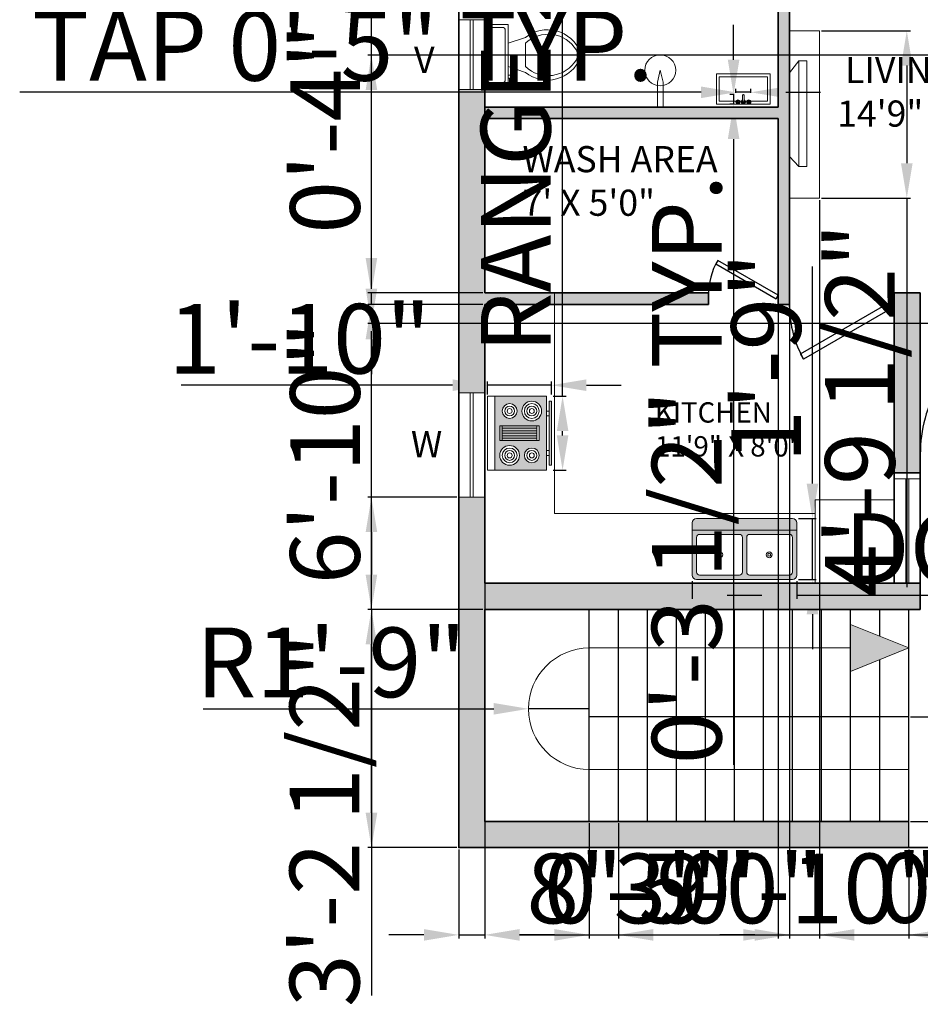
# Model space of a CAD drawing. Units: inches. Extents: x 830 to 1639, y 2591 to 3595.
# Tile 1 of 7: x 830 to 1141, y 2618 to 2957. Entities that reach past the tile are written whole.
import ezdxf

# ---------------------------------------------------------------- set-up
doc = ezdxf.new("R2010")
doc.units = ezdxf.units.IN
doc.layers.get('0').update_dxf_attribs({"color": 250})
for name, color, linetype, lineweight in [('A-ANNO-DIMS', 2, 'Continuous', 18), ('A-ANNO-SYMB', 2, 'Continuous', 18), ('A-ANNO-TEXT', 7, 'Continuous', 18), ('A-AREA-IDEN', 7, 'Continuous', 25), ('A-DOOR', 3, 'Continuous', 25), ('A-EQPM', 9, 'Continuous', 18), ('A-FLOR-CASE', 8, 'Continuous', 18), ('A-FLOR-FIXT', 8, 'Continuous', 18), ('A-FLOR-FIXT-PATT', 30, 'Continuous', 13), ('A-FLOR-STRS', 7, 'Continuous', 25), ('A-FURN', 8, 'Continuous', 18), ('A-GLAZ', 4, 'Continuous', 18), ('A-WALL', 7, 'Continuous', 35), ('A-WALL-PATT', 5, 'Continuous', 13), ('C-PROP', 7, 'Continuous', 35)]:
    doc.layers.add(name, color=color, linetype=linetype, lineweight=lineweight)
doc.styles.get("Standard").update_dxf_attribs({"font": 'arial.ttf'})
doc.dimstyles.new('ISO-25', dxfattribs={"dimtxt": 24, "dimasz": 12, "dimexe": 1.25, "dimexo": 0.625, "dimtad": 1, "dimdec": 0, "dimlunit": 3, "dimtxsty": 'Standard', "dimcen": 2.5, "dimadec": 0, "dimazin": 0, "dimtfac": 1, "dimtdec": 0, "dimtmove": 0, "dimatfit": 3, "dimfxl": 1, "dimarcsym": 0})

# ---------------------------------------------------------------- blocks, each defined once
blk = doc.blocks.new('Sink-double - 36 in top')
for p, q in [((-18, -4), (18, -4)), ((-0.75, -18.5), (-0.75, -6.5)), ((0.75, -6.5), (0.75, -18.5))]:
    blk.add_line(p, q)
for points in [[(-16.5, 0), (16.5, 0)], [(-18, -19.5), (-18, -1.5)], [(18, -1.5), (18, -19.5)], [(-16.5, -18.5), (-16.5, -6.5)], [(-15.5, -5.5), (-1.75, -5.5)], [(1.75, -5.5), (15.5, -5.5)], [(16.5, -6.5), (16.5, -18.5)], [(-1.75, -19.5), (-15.5, -19.5)], [(15.5, -19.5), (1.75, -19.5)], [(16.5, -21), (-16.5, -21)]]:
    blk.add_lwpolyline(points)
for centre, radius in [((-8.5, -12.5), 1), ((-8.5, -12.5), 0.5), ((8.5, -12.5), 1), ((8.5, -12.5), 0.5)]:
    blk.add_circle(centre, radius)
for centre, radius, start, end in [((-16.5, -1.5), 1.5, 90, 180), ((16.5, -1.5), 1.5, 0, 90), ((-15.5, -6.5), 1, 90, 180), ((-1.75, -6.5), 1, 0, 90), ((1.75, -6.5), 1, 90, 180), ((15.5, -6.5), 1, 0, 90), ((-16.5, -19.5), 1.5, 180, 270), ((-15.5, -18.5), 1, 180, 270), ((-1.75, -18.5), 1, 270, 0), ((1.75, -18.5), 1, 180, 270), ((15.5, -18.5), 1, 270, 0), ((16.5, -19.5), 1.5, 270, 0)]:
    blk.add_arc(centre, radius, start, end)
blk = doc.blocks.new('Toilet - top')
for p, q in [((9.5, -6), (9.5, -2)), ((-10, -8.5), (-8, -8.5)), ((-10, -9.5), (-10, -8.5)), ((-7, -9.5), (-10, -9.5)), ((-8, -8.5), (-8, -8)), ((-7, -8), (-7, -9.5)), ((-4, -8), (-6, -14)), ((4, -8), (6, -14)), ((4, -14), (-4, -14))]:
    blk.add_line(p, q)
blk.add_lwpolyline([(10.5, -8), (10.5, 0), (-10.5, 0), (-10.5, -8)], close=True)
for points in [[(-9.5, -2), (-9.5, -6)], [(8.5, -1), (-8.5, -1)], [(-8.5, -7), (8.5, -7)]]:
    blk.add_lwpolyline(points)
for centre, radius, start, end in [((-8.62, -1.88), 0.884, 81.8699, 188.1301), ((8.62, -1.88), 0.884, 351.8699, 98.1301), ((-8.62, -6.12), 0.884, 171.8699, 278.1301), ((8.62, -6.12), 0.884, 261.8699, 8.1301), ((3.52, -21.58), 12.17, 141.4691, 247.9714), ((4.2, -21.82), 11.33, 136.3677, 238.9468), ((-3.52, -21.58), 12.17, 292.0284, 38.5307), ((-4.2, -21.82), 11.33, 301.053, 43.6321), ((0, -27.88), 4, 245.7318, 294.2682), ((0, -29), 4, 254.8605, 285.1395)]:
    blk.add_arc(centre, radius, start, end)
blk = doc.blocks.new('*U9')
for p, q in [((-750, 0), (-750, -100)), ((0, 0), (0, -100))]:
    blk.add_line(p, q)
blk.add_lwpolyline([(0, 0), (-649.5, 375), (-671.4, 337.1), (-21.9, -37.9)], close=True)
blk.add_arc((0, 0), 750, 150, 180)
blk = doc.blocks.new('*U12')
for p, q in [((0, 0), (0, -100)), ((750, 0), (750, -100))]:
    blk.add_line(p, q)
blk.add_lwpolyline([(0, 0), (649.5, 375), (671.4, 337.1), (21.9, -37.9)], close=True)
blk.add_arc((0, 0), 750, 0, 30)
blk = doc.blocks.new('Range-Oven - 30 in top')
for p, q in [((0, -3), (30, -3)), ((12, -6), (18, -6)), ((13, -20), (13, -6)), ((14, -6), (14, -20)), ((15, -20), (15, -6)), ((16, -6), (16, -20)), ((17, -20), (17, -6)), ((18, -20), (12, -20)), ((6, -24), (6, -25)), ((8, -25), (8, -24)), ((22, -25), (22, -24)), ((24, -24), (24, -25))]:
    blk.add_line(p, q)
for points in [[(0, -24), (0, 0), (30, 0), (30, -24)], [(12, -21), (12, -5), (18, -5), (18, -21)], [(2, -26), (2, -25), (28, -25), (28, -26)]]:
    blk.add_lwpolyline(points, close=True)
for centre, radius in [((6, -9), 4), ((6, -9), 3), ((6, -9), 2), ((24, -9), 3), ((24, -9), 2), ((6, -9), 1), ((24, -9), 1), ((6, -18), 3), ((24, -18), 4), ((24, -18), 3), ((6, -18), 2), ((6, -18), 1), ((24, -18), 2), ((24, -18), 1)]:
    blk.add_circle(centre, radius)
blk = doc.blocks.new('Faucet - Bathroom top')
for p, q in [((-4.107, 0.125), (-4.375, 0.125)), ((-3.75, 0.4788), (-3.75, 0.75)), ((-3.5, 0.482), (-3.5, 0.75)), ((-3.1461, 0.125), (-2.875, 0.125)), ((3.143, 0.125), (2.875, 0.125)), ((3.5, 0.4788), (3.5, 0.75)), ((3.75, 0.482), (3.75, 0.75)), ((4.1039, 0.125), (4.375, 0.125)), ((-4.1039, -0.125), (-4.375, -0.125)), ((-3.75, -0.4821), (-3.75, -0.75)), ((-3.5, -0.4789), (-3.5, -0.75)), ((-3.143, -0.125), (-2.875, -0.125)), ((-0.5, -0.8639), (-0.5, -4.5)), ((0.5, -4.5), (0.5, -0.8631)), ((3.1461, -0.125), (2.875, -0.125)), ((3.5, -0.4821), (3.5, -0.75)), ((3.75, -0.4789), (3.75, -0.75)), ((4.107, -0.125), (4.375, -0.125))]:
    blk.add_line(p, q)
for centre, radius in [((-3.625, 0), 1.375), ((-4.625, 0), 0.2795), ((-3.625, 0), 0.5), ((-3.625, 1), 0.2795), ((-2.625, 0), 0.2795), ((0, 0), 0.5), ((3.625, 0), 1.375), ((2.625, 0), 0.2795), ((3.625, 0), 0.5), ((3.625, 1), 0.2795), ((4.625, 0), 0.2795), ((-3.625, -1), 0.2795), ((3.625, -1), 0.2795)]:
    blk.add_circle(centre, radius)
for centre, radius, start, end in [((-3.625, 0), 1, 105.2407, 164.2093), ((-3.625, 0), 1, 16.44125, 74.07887), ((0, 0), 1.5, 289.6514, 250.3603), ((0, 0), 1, 300.3431, 239.7554), ((3.625, 0), 1, 106.12, 164.0884), ((3.625, 0), 1, 16.23422, 73.90469), ((-3.625, 0), 1, 196.2342, 253.9047), ((-3.625, 0), 1, 286.12, 344.0884), ((0, -4.5), 0.5, 180, 0), ((3.625, 0), 1, 196.4413, 254.0789), ((3.625, 0), 1, 285.2407, 344.2093)]:
    blk.add_arc(centre, radius, start, end)
blk = doc.blocks.new('WIN-36IN')
for p, q in [((0, 0), (0, 36)), ((0, 36), (9, 36)), ((4, 0), (4, 36)), ((5, 36), (5, 0)), ((9, 36), (9, 0)), ((9, 0), (0, 0))]:
    blk.add_line(p, q)
blk = doc.blocks.new('VENT-24IN')
for p, q in [((0, 24), (9, 24)), ((0, 0), (0, 24)), ((4, 0), (4, 24)), ((5, 24), (5, 0)), ((9, 24), (9, 0)), ((9, 0), (0, 0))]:
    blk.add_line(p, q)
blk = doc.blocks.new('LAVATORY-RECT')
for points in [[(0, 10.45), (18.57, 10.45), (18.57, 0), (0, 0)], [(1, 9.45), (17.57, 9.45), (17.57, 1), (1, 1)]]:
    blk.add_lwpolyline(points, close=True)
blk = doc.blocks.new('SHOWER-HEAD-PLAN')
for p, q in [((4.38, 8.59), (5.33, 12.63)), ((5.33, 12.63), (6.38, 8.59)), ((4.38, 0), (4.38, 8.59)), ((6.38, 0), (6.38, 8.59))]:
    blk.add_line(p, q)
blk.add_circle((5.33, 12.63), 5.33)
blk = doc.blocks.new('*D32')
at = {"layer": 'A-ANNO-DIMS', "color": 0, "lineweight": -2, "transparency": 16777216}
for p, q in [((1077.06, 2932), (1077.06, 2933.4)), ((1082.22, 2932), (1082.22, 2933.4)), ((1065.06, 2932.15), (830.39, 2932.15)), ((1082.22, 2932.15), (1077.06, 2932.15)), ((1094.22, 2932.15), (1106.22, 2932.15))]:
    blk.add_line(p, q, dxfattribs=at)
at = {"layer": 'A-ANNO-DIMS', "color": 0, "transparency": 16777216}
for points in [[(1065.06, 2934.15), (1065.06, 2930.15), (1077.06, 2932.15)], [(1094.22, 2934.15), (1094.22, 2930.15), (1082.22, 2932.15)]]:
    blk.add_solid(points, dxfattribs=at)
at = {"layer": 'Defpoints', "color": 0, "transparency": 16777216}
for p in [(1077.06, 2932.15), (1077.06, 2931.38), (1082.22, 2931.38)]:
    blk.add_point(p, dxfattribs=at)
at = {"layer": 'A-ANNO-DIMS', "color": 0, "transparency": 16777216, "insert": (941.72, 2945.03), "char_height": 24, "attachment_point": 5}
blk.add_mtext('TAP 0\'-5" TYP.', dxfattribs=at)
blk = doc.blocks.new('*D33')
at = {"layer": 'A-ANNO-DIMS', "color": 0, "lineweight": -2, "transparency": 16777216}
for p, q in [((1076.28, 2943.38), (1076.28, 2955.38)), ((1076.43, 2931.38), (1075.03, 2931.38)), ((1076.28, 2931.38), (1076.28, 2928.02)), ((1076.43, 2928.02), (1075.03, 2928.02)), ((1076.28, 2916.02), (1076.28, 2700.56))]:
    blk.add_line(p, q, dxfattribs=at)
at = {"layer": 'A-ANNO-DIMS', "color": 0, "transparency": 16777216}
for points in [[(1074.28, 2943.38), (1078.28, 2943.38), (1076.28, 2931.38)], [(1074.28, 2916.02), (1078.28, 2916.02), (1076.28, 2928.02)]]:
    blk.add_solid(points, dxfattribs=at)
at = {"layer": 'Defpoints', "color": 0, "transparency": 16777216}
for p in [(1077.06, 2931.38), (1076.28, 2928.02), (1077.06, 2928.02)]:
    blk.add_point(p, dxfattribs=at)
at = {"layer": 'A-ANNO-DIMS', "color": 0, "transparency": 16777216, "insert": (1063.24, 2802.29), "char_height": 24, "attachment_point": 5, "rotation": 90}
blk.add_mtext('0\'-3 1/2" TYP.', dxfattribs=at)
blk = doc.blocks.new('*D42')
at = {"layer": 'A-ANNO-DIMS', "color": 0, "lineweight": -2, "transparency": 16777216}
for p, q in [((1062.05, 2763.79), (1062.05, 2757.77)), ((1098.05, 2763.79), (1098.05, 2757.77)), ((1074.05, 2759.02), (1086.05, 2759.02)), ((1098.05, 2759.02), (1408.67, 2759.02))]:
    blk.add_line(p, q, dxfattribs=at)
at = {"layer": 'A-ANNO-DIMS', "color": 0, "transparency": 16777216}
for points in [[(1074.05, 2761.02), (1074.05, 2757.02), (1062.05, 2759.02)], [(1086.05, 2761.02), (1086.05, 2757.02), (1098.05, 2759.02)]]:
    blk.add_solid(points, dxfattribs=at)
at = {"layer": 'Defpoints', "color": 0, "transparency": 16777216}
for p in [(1062.05, 2764.42), (1098.05, 2764.42), (1098.05, 2759.02)]:
    blk.add_point(p, dxfattribs=at)
at = {"layer": 'A-ANNO-DIMS', "color": 0, "transparency": 16777216, "insert": (1259.36, 2772.07), "char_height": 24, "attachment_point": 5}
blk.add_mtext('DOUBLE SINK 3\'-0"', dxfattribs=at)
blk = doc.blocks.new('*D43')
at = {"layer": 'A-ANNO-DIMS', "color": 0, "lineweight": -2, "transparency": 16777216}
for p, q in [((1103.45, 2797.42), (1103.45, 2872.21)), ((1098.68, 2785.42), (1104.7, 2785.42)), ((1103.45, 2764.42), (1103.45, 2785.42)), ((1098.68, 2764.42), (1104.7, 2764.42)), ((1103.45, 2752.42), (1103.45, 2740.42))]:
    blk.add_line(p, q, dxfattribs=at)
at = {"layer": 'A-ANNO-DIMS', "color": 0, "transparency": 16777216}
for points in [[(1101.45, 2797.42), (1105.45, 2797.42), (1103.45, 2785.42)], [(1101.45, 2752.42), (1105.45, 2752.42), (1103.45, 2764.42)]]:
    blk.add_solid(points, dxfattribs=at)
at = {"layer": 'Defpoints', "color": 0, "transparency": 16777216}
for p in [(1098.05, 2785.42), (1103.45, 2785.42), (1098.05, 2764.42)]:
    blk.add_point(p, dxfattribs=at)
at = {"layer": 'A-ANNO-DIMS', "color": 0, "transparency": 16777216, "insert": (1090.57, 2840.81), "char_height": 24, "attachment_point": 5, "rotation": 90}
blk.add_mtext('1\'-9"', dxfattribs=at)
blk = doc.blocks.new('*D44')
at = {"layer": 'A-ANNO-DIMS', "color": 0, "lineweight": -2, "transparency": 16777216}
for p, q in [((1017.38, 2827.49), (1017.38, 3087.77)), ((1014.18, 2827.49), (1018.63, 2827.49)), ((1017.38, 2814.04), (1017.38, 2815.49)), ((1014.18, 2802.04), (1018.63, 2802.04))]:
    blk.add_line(p, q, dxfattribs=at)
at = {"layer": 'A-ANNO-DIMS', "color": 0, "transparency": 16777216}
for points in [[(1015.38, 2815.49), (1019.38, 2815.49), (1017.38, 2827.49)], [(1015.38, 2814.04), (1019.38, 2814.04), (1017.38, 2802.04)]]:
    blk.add_solid(points, dxfattribs=at)
at = {"layer": 'Defpoints', "color": 0, "transparency": 16777216}
for p in [(1013.56, 2827.49), (1017.38, 2827.49), (1013.56, 2802.04)]:
    blk.add_point(p, dxfattribs=at)
at = {"layer": 'A-ANNO-DIMS', "color": 0, "transparency": 16777216, "insert": (1004.34, 2963.63), "char_height": 24, "attachment_point": 5, "rotation": 90}
blk.add_mtext('RANGE 2\'-1 1/2"', dxfattribs=at)
blk = doc.blocks.new('*D45')
at = {"layer": 'A-ANNO-DIMS', "color": 0, "lineweight": -2, "transparency": 16777216}
for p, q in [((979.5, 2831.31), (886.06, 2831.31)), ((991.5, 2828.12), (991.5, 2832.56)), ((1013.56, 2831.31), (991.5, 2831.31)), ((1013.56, 2828.12), (1013.56, 2832.56)), ((1025.56, 2831.31), (1037.56, 2831.31))]:
    blk.add_line(p, q, dxfattribs=at)
at = {"layer": 'A-ANNO-DIMS', "color": 0, "transparency": 16777216}
for points in [[(979.5, 2833.31), (979.5, 2829.31), (991.5, 2831.31)], [(1025.56, 2833.31), (1025.56, 2829.31), (1013.56, 2831.31)]]:
    blk.add_solid(points, dxfattribs=at)
at = {"layer": 'Defpoints', "color": 0, "transparency": 16777216}
for p in [(991.5, 2831.31), (991.5, 2827.49), (1013.56, 2827.49)]:
    blk.add_point(p, dxfattribs=at)
at = {"layer": 'A-ANNO-DIMS', "color": 0, "transparency": 16777216, "insert": (926.78, 2844.19), "char_height": 24, "attachment_point": 5}
blk.add_mtext('1\'-10"', dxfattribs=at)
blk = doc.blocks.new('*D46')
at = {"layer": 'A-ANNO-DIMS', "color": 0, "lineweight": -2, "transparency": 16777216}
for p, q in [((1136.59, 2671.46), (1136.59, 2640.79)), ((1272.59, 2671.46), (1272.59, 2640.79)), ((1148.59, 2642.04), (1260.59, 2642.04))]:
    blk.add_line(p, q, dxfattribs=at)
at = {"layer": 'A-ANNO-DIMS', "color": 0, "transparency": 16777216}
for points in [[(1148.59, 2644.04), (1148.59, 2640.04), (1136.59, 2642.04)], [(1260.59, 2644.04), (1260.59, 2640.04), (1272.59, 2642.04)]]:
    blk.add_solid(points, dxfattribs=at)
at = {"layer": 'Defpoints', "color": 0, "transparency": 16777216}
for p in [(1136.59, 2672.09), (1272.59, 2672.09), (1272.59, 2642.04)]:
    blk.add_point(p, dxfattribs=at)
at = {"layer": 'A-ANNO-DIMS', "color": 0, "transparency": 16777216, "insert": (1204.59, 2654.71), "char_height": 24, "attachment_point": 5}
blk.add_mtext('11\'-4"', dxfattribs=at)
blk = doc.blocks.new('*D47')
at = {"layer": 'A-ANNO-DIMS', "color": 0, "lineweight": -2, "transparency": 16777216}
for p, q in [((951.54, 2754.09), (951.54, 2849.91)), ((989.96, 2754.09), (950.29, 2754.09)), ((951.54, 2684.09), (951.54, 2742.09)), ((980.96, 2672.09), (950.29, 2672.09))]:
    blk.add_line(p, q, dxfattribs=at)
at = {"layer": 'A-ANNO-DIMS', "color": 0, "transparency": 16777216}
for points in [[(949.54, 2742.09), (953.54, 2742.09), (951.54, 2754.09)], [(949.54, 2684.09), (953.54, 2684.09), (951.54, 2672.09)]]:
    blk.add_solid(points, dxfattribs=at)
at = {"layer": 'Defpoints', "color": 0, "transparency": 16777216}
for p in [(951.54, 2754.09), (990.59, 2754.09), (981.59, 2672.09)]:
    blk.add_point(p, dxfattribs=at)
at = {"layer": 'A-ANNO-DIMS', "color": 0, "transparency": 16777216, "insert": (938.66, 2808), "char_height": 24, "attachment_point": 5, "rotation": 90}
blk.add_mtext('6\'-10"', dxfattribs=at)
blk = doc.blocks.new('*D51')
at = {"layer": 'A-ANNO-DIMS', "color": 0, "lineweight": -2, "transparency": 16777216}
for p, q in [((990.59, 2680.46), (990.59, 2640.79)), ((981.59, 2671.46), (981.59, 2640.79)), ((969.59, 2642.04), (957.59, 2642.04)), ((981.59, 2642.04), (990.59, 2642.04)), ((1002.59, 2642.04), (1079.64, 2642.04))]:
    blk.add_line(p, q, dxfattribs=at)
at = {"layer": 'A-ANNO-DIMS', "color": 0, "transparency": 16777216}
for points in [[(969.59, 2644.04), (969.59, 2640.04), (981.59, 2642.04)], [(1002.59, 2644.04), (1002.59, 2640.04), (990.59, 2642.04)]]:
    blk.add_solid(points, dxfattribs=at)
at = {"layer": 'Defpoints', "color": 0, "transparency": 16777216}
for p in [(990.59, 2681.09), (981.59, 2672.09), (990.59, 2642.04)]:
    blk.add_point(p, dxfattribs=at)
at = {"layer": 'A-ANNO-DIMS', "color": 0, "transparency": 16777216, "insert": (1047.11, 2654.92), "char_height": 24, "attachment_point": 5}
blk.add_mtext('0\'-9"', dxfattribs=at)
blk = doc.blocks.new('*D52')
at = {"layer": 'A-ANNO-DIMS', "color": 0, "lineweight": -2, "transparency": 16777216}
for p, q in [((951.54, 2875.09), (951.54, 2952.14)), ((989.96, 2863.09), (950.29, 2863.09)), ((951.54, 2859.09), (951.54, 2863.09)), ((989.96, 2859.09), (950.29, 2859.09)), ((951.54, 2847.09), (951.54, 2835.09))]:
    blk.add_line(p, q, dxfattribs=at)
at = {"layer": 'A-ANNO-DIMS', "color": 0, "transparency": 16777216}
for points in [[(949.54, 2875.09), (953.54, 2875.09), (951.54, 2863.09)], [(949.54, 2847.09), (953.54, 2847.09), (951.54, 2859.09)]]:
    blk.add_solid(points, dxfattribs=at)
at = {"layer": 'Defpoints', "color": 0, "transparency": 16777216}
for p in [(951.54, 2863.09), (990.59, 2863.09), (990.59, 2859.09)]:
    blk.add_point(p, dxfattribs=at)
at = {"layer": 'A-ANNO-DIMS', "color": 0, "transparency": 16777216, "insert": (938.66, 2919.61), "char_height": 24, "attachment_point": 5, "rotation": 90}
blk.add_mtext('0\'-4"', dxfattribs=at)
blk = doc.blocks.new('*D53')
at = {"layer": 'A-ANNO-DIMS', "color": 0, "lineweight": -2, "transparency": 16777216}
for p, q in [((1026.59, 2680.46), (1026.59, 2640.79)), ((1036.59, 2680.46), (1036.59, 2640.79)), ((1014.59, 2642.04), (1002.59, 2642.04)), ((1026.59, 2642.04), (1036.59, 2642.04)), ((1048.59, 2642.04), (1144.28, 2642.04))]:
    blk.add_line(p, q, dxfattribs=at)
at = {"layer": 'A-ANNO-DIMS', "color": 0, "transparency": 16777216}
for points in [[(1014.59, 2644.04), (1014.59, 2640.04), (1026.59, 2642.04)], [(1048.59, 2644.04), (1048.59, 2640.04), (1036.59, 2642.04)]]:
    blk.add_solid(points, dxfattribs=at)
at = {"layer": 'Defpoints', "color": 0, "transparency": 16777216}
for p in [(1026.59, 2681.09), (1036.59, 2681.09), (1036.59, 2642.04)]:
    blk.add_point(p, dxfattribs=at)
at = {"layer": 'A-ANNO-DIMS', "color": 0, "transparency": 16777216, "insert": (1102.44, 2654.92), "char_height": 24, "attachment_point": 5}
blk.add_mtext('0\'-10"', dxfattribs=at)
blk = doc.blocks.new('*D54')
at = {"layer": 'A-ANNO-DIMS', "color": 0, "lineweight": -2, "transparency": 16777216}
for p, q in [((990.59, 2680.46), (990.59, 2640.79)), ((1026.59, 2680.46), (1026.59, 2640.79)), ((1002.59, 2642.04), (1014.59, 2642.04)), ((1026.59, 2642.04), (1103.62, 2642.04))]:
    blk.add_line(p, q, dxfattribs=at)
at = {"layer": 'A-ANNO-DIMS', "color": 0, "transparency": 16777216}
for points in [[(1002.59, 2644.04), (1002.59, 2640.04), (990.59, 2642.04)], [(1014.59, 2644.04), (1014.59, 2640.04), (1026.59, 2642.04)]]:
    blk.add_solid(points, dxfattribs=at)
at = {"layer": 'Defpoints', "color": 0, "transparency": 16777216}
for p in [(990.59, 2681.09), (1026.59, 2681.09), (1026.59, 2642.04)]:
    blk.add_point(p, dxfattribs=at)
at = {"layer": 'A-ANNO-DIMS', "color": 0, "transparency": 16777216, "insert": (1071.11, 2654.92), "char_height": 24, "attachment_point": 5}
blk.add_mtext('3\'-0"', dxfattribs=at)
blk = doc.blocks.new('*D55')
at = {"layer": 'A-ANNO-DIMS', "color": 0, "lineweight": -2, "transparency": 16777216}
for p, q in [((1311.64, 2717.09), (1311.64, 2794.12)), ((1137.21, 2717.09), (1312.89, 2717.09)), ((1311.64, 2693.09), (1311.64, 2705.09)), ((1137.21, 2681.09), (1312.89, 2681.09))]:
    blk.add_line(p, q, dxfattribs=at)
at = {"layer": 'A-ANNO-DIMS', "color": 0, "transparency": 16777216}
for points in [[(1309.64, 2705.09), (1313.64, 2705.09), (1311.64, 2717.09)], [(1309.64, 2693.09), (1313.64, 2693.09), (1311.64, 2681.09)]]:
    blk.add_solid(points, dxfattribs=at)
at = {"layer": 'Defpoints', "color": 0, "transparency": 16777216}
for p in [(1136.59, 2717.09), (1311.64, 2717.09), (1136.59, 2681.09)]:
    blk.add_point(p, dxfattribs=at)
at = {"layer": 'A-ANNO-DIMS', "color": 0, "transparency": 16777216, "insert": (1298.75, 2761.6), "char_height": 24, "attachment_point": 5, "rotation": 90}
blk.add_mtext('3\'-0"', dxfattribs=at)
blk = doc.blocks.new('*D57')
at = {"layer": 'A-ANNO-DIMS', "color": 0, "lineweight": -2, "transparency": 16777216}
for p, q in [((951.54, 2944.9), (951.54, 3077.67)), ((1203.59, 2944.9), (950.29, 2944.9)), ((951.54, 2864.53), (951.54, 2932.9)), ((1203.59, 2852.53), (950.29, 2852.53))]:
    blk.add_line(p, q, dxfattribs=at)
at = {"layer": 'A-ANNO-DIMS', "color": 0, "transparency": 16777216}
for points in [[(949.54, 2932.9), (953.54, 2932.9), (951.54, 2944.9)], [(949.54, 2864.53), (953.54, 2864.53), (951.54, 2852.53)]]:
    blk.add_solid(points, dxfattribs=at)
at = {"layer": 'Defpoints', "color": 0, "transparency": 16777216}
for p in [(951.54, 2944.9), (1204.22, 2944.9), (1204.22, 2852.53)]:
    blk.add_point(p, dxfattribs=at)
at = {"layer": 'A-ANNO-DIMS', "color": 0, "transparency": 16777216, "insert": (938.51, 3017.28), "char_height": 24, "attachment_point": 5, "rotation": 90}
blk.add_mtext('7\'-8 1/2"', dxfattribs=at)
blk = doc.blocks.new('*D59')
at = {"layer": 'A-ANNO-DIMS', "color": 0, "lineweight": -2, "transparency": 16777216}
for p, q in [((990.59, 2858.46), (990.59, 2640.79)), ((1091.59, 2858.46), (1091.59, 2640.79)), ((1002.59, 2642.04), (1079.59, 2642.04))]:
    blk.add_line(p, q, dxfattribs=at)
at = {"layer": 'A-ANNO-DIMS', "color": 0, "transparency": 16777216}
for points in [[(1002.59, 2644.04), (1002.59, 2640.04), (990.59, 2642.04)], [(1079.59, 2644.04), (1079.59, 2640.04), (1091.59, 2642.04)]]:
    blk.add_solid(points, dxfattribs=at)
at = {"layer": 'Defpoints', "color": 0, "transparency": 16777216}
for p in [(990.59, 2859.09), (1091.59, 2859.09), (1091.59, 2642.04)]:
    blk.add_point(p, dxfattribs=at)
at = {"layer": 'A-ANNO-DIMS', "color": 0, "transparency": 16777216, "insert": (1041.09, 2654.92), "char_height": 24, "attachment_point": 5}
blk.add_mtext('8\'-5"', dxfattribs=at)
blk = doc.blocks.new('*D60')
at = {"layer": 'A-ANNO-DIMS', "color": 0, "lineweight": -2, "transparency": 16777216}
for p, q in [((980.96, 2792.71), (950.29, 2792.71)), ((951.54, 2780.71), (951.54, 2766.09)), ((989.96, 2754.09), (950.29, 2754.09)), ((951.54, 2754.09), (951.54, 2621.13))]:
    blk.add_line(p, q, dxfattribs=at)
at = {"layer": 'A-ANNO-DIMS', "color": 0, "transparency": 16777216}
for points in [[(949.54, 2780.71), (953.54, 2780.71), (951.54, 2792.71)], [(949.54, 2766.09), (953.54, 2766.09), (951.54, 2754.09)]]:
    blk.add_solid(points, dxfattribs=at)
at = {"layer": 'Defpoints', "color": 0, "transparency": 16777216}
for p in [(981.59, 2792.71), (951.54, 2754.09), (990.59, 2754.09)]:
    blk.add_point(p, dxfattribs=at)
at = {"layer": 'A-ANNO-DIMS', "color": 0, "transparency": 16777216, "insert": (938.5, 2681.61), "char_height": 24, "attachment_point": 5, "rotation": 90}
blk.add_mtext('3\'-2 1/2"', dxfattribs=at)
blk = doc.blocks.new('*D64')
at = {"layer": 'A-ANNO-DIMS', "color": 0, "lineweight": -2, "transparency": 16777216}
for p, q in [((1095.59, 2895.07), (1095.59, 2640.79)), ((1105.88, 2895.07), (1105.88, 2640.79)), ((1083.59, 2642.04), (1071.59, 2642.04)), ((1095.59, 2642.04), (1105.88, 2642.04)), ((1117.88, 2642.04), (1269.5, 2642.04))]:
    blk.add_line(p, q, dxfattribs=at)
at = {"layer": 'A-ANNO-DIMS', "color": 0, "transparency": 16777216}
for points in [[(1083.59, 2644.04), (1083.59, 2640.04), (1095.59, 2642.04)], [(1117.88, 2644.04), (1117.88, 2640.04), (1105.88, 2642.04)]]:
    blk.add_solid(points, dxfattribs=at)
at = {"layer": 'Defpoints', "color": 0, "transparency": 16777216}
for p in [(1095.59, 2895.7), (1105.88, 2895.7), (1105.88, 2642.04)]:
    blk.add_point(p, dxfattribs=at)
at = {"layer": 'A-ANNO-DIMS', "color": 0, "transparency": 16777216, "insert": (1199.69, 2655.07), "char_height": 24, "attachment_point": 5}
blk.add_mtext('0\'-10 1/2"', dxfattribs=at)
blk = doc.blocks.new('*D65')
at = {"layer": 'A-ANNO-DIMS', "color": 0, "lineweight": -2, "transparency": 16777216}
for p, q in [((1106.51, 2953.33), (1137.18, 2953.33)), ((1135.93, 2941.33), (1135.93, 2907.7)), ((1106.51, 2895.7), (1137.18, 2895.7)), ((1135.93, 2895.7), (1135.93, 2761.76))]:
    blk.add_line(p, q, dxfattribs=at)
at = {"layer": 'A-ANNO-DIMS', "color": 0, "transparency": 16777216}
for points in [[(1133.93, 2941.33), (1137.93, 2941.33), (1135.93, 2953.33)], [(1133.93, 2907.7), (1137.93, 2907.7), (1135.93, 2895.7)]]:
    blk.add_solid(points, dxfattribs=at)
at = {"layer": 'Defpoints', "color": 0, "transparency": 16777216}
for p in [(1105.88, 2953.33), (1105.88, 2895.7), (1135.93, 2895.7)]:
    blk.add_point(p, dxfattribs=at)
at = {"layer": 'A-ANNO-DIMS', "color": 0, "transparency": 16777216, "insert": (1122.9, 2822.73), "char_height": 24, "attachment_point": 5, "rotation": 90}
blk.add_mtext('4\'-9 1/2"', dxfattribs=at)
blk = doc.blocks.new('*D78')
at = {"layer": 'A-ANNO-DIMS', "color": 0, "lineweight": -2, "transparency": 16777216}
for p, q in [((893.64, 2719.88), (993.65, 2719.88)), ((1026.59, 2719.89), (1005.65, 2719.88))]:
    blk.add_line(p, q, dxfattribs=at)
at = {"layer": 'A-ANNO-DIMS', "color": 0, "transparency": 16777216}
blk.add_solid([(993.65, 2721.88), (993.65, 2717.88), (1005.65, 2719.88)], dxfattribs=at)
at = {"layer": 'Defpoints', "color": 0, "transparency": 16777216}
for p in [(1005.65, 2719.88), (1026.59, 2719.89)]:
    blk.add_point(p, dxfattribs=at)
at = {"layer": 'A-ANNO-DIMS', "color": 0, "transparency": 16777216, "insert": (937.65, 2732.76), "char_height": 24, "attachment_point": 5, "rotation": 0.0003}
blk.add_mtext('R1\'-9"', dxfattribs=at)

msp = doc.modelspace()

# ---------------------------------------------------------------- hatches: boundary and pattern name
at = {"layer": 'A-ANNO-SYMB'}
h = msp.add_hatch(color=256, dxfattribs=at)
h.dxf.hatch_style = 1
h.paths.add_polyline_path([(1136.59, 2740.82), (1116.59, 2748.87), (1116.59, 2732.77)])
at = {"layer": 'A-FLOR-FIXT-PATT'}
h = msp.add_hatch(color=256, dxfattribs=at)
h.dxf.hatch_style = 1
h.paths.add_polyline_path([(1009.31, 2817.31), (1008.47, 2817.31), (1008.47, 2812.22), (1009.31, 2812.22)], flags=16)
h.paths.add_polyline_path([(996.59, 2822.4, -1), (1001.68, 2822.4, -1)], flags=16)
h.paths.add_polyline_path([(997.44, 2822.4, -1), (1000.83, 2822.4, -1)], flags=0)
h.paths.add_polyline_path([(1003.37, 2822.4, -1), (1010.16, 2822.4, -1)], flags=16)
h.paths.add_polyline_path([(998.28, 2822.4, -1), (999.98, 2822.4, -1)], flags=0)
h.paths.add_polyline_path([(1004.22, 2822.4, -1), (1009.31, 2822.4, -1)], flags=0)
h.paths.add_polyline_path([(1005.07, 2822.4, -1), (1008.47, 2822.4, -1)], flags=0)
h.paths.add_polyline_path([(1005.92, 2822.4, -1), (1007.62, 2822.4, -1)], flags=0)
h.paths.add_polyline_path([(994.04, 2802.04), (1011.86, 2802.04), (1011.86, 2827.49), (994.04, 2827.49)])
h.paths.add_polyline_path([(1002.53, 2807.13, -1), (995.74, 2807.13, -1)], flags=16)
h.paths.add_polyline_path([(1001.68, 2807.13, -1), (996.59, 2807.13, -1)], flags=0)
h.paths.add_polyline_path([(1000.83, 2807.13, -1), (997.44, 2807.13, -1)], flags=0)
h.paths.add_polyline_path([(1009.31, 2807.13, -1), (1004.22, 2807.13, -1)], flags=16)
h.paths.add_polyline_path([(999.98, 2807.13, -1), (998.28, 2807.13, -1)], flags=0)
h.paths.add_polyline_path([(1008.47, 2807.13, -1), (1005.07, 2807.13, -1)], flags=0)
h.paths.add_polyline_path([(1012.71, 2825.8), (1013.56, 2825.8), (1013.56, 2803.73), (1012.71, 2803.73)])
h.paths.add_polyline_path([(1007.62, 2807.13, -1), (1005.92, 2807.13, -1)], flags=0)
h = msp.add_hatch(color=256, dxfattribs=at)
h.dxf.hatch_style = 1
h.paths.add_polyline_path([(1098.05, 2781.42), (1098.05, 2783.92, 0.414214), (1096.55, 2785.42), (1063.55, 2785.42, 0.414214), (1062.05, 2783.92), (1062.05, 2781.42)])
h = msp.add_hatch(color=256, dxfattribs=at)
h.dxf.hatch_style = 1
h.paths.add_polyline_path([(1081.8, 2779.92, 0.414214), (1080.8, 2778.92), (1080.8, 2766.92, 0.414214), (1081.8, 2765.92), (1095.55, 2765.92, 0.414214), (1096.55, 2766.92), (1096.55, 2778.92, 0.414214), (1095.55, 2779.92)], flags=16)
h.paths.add_polyline_path([(1062.05, 2781.42), (1062.05, 2765.92, 0.414214), (1063.55, 2764.42), (1096.55, 2764.42, 0.414214), (1098.05, 2765.92), (1098.05, 2781.42)])
h.paths.add_polyline_path([(1079.3, 2778.92), (1079.3, 2766.92, -0.414214), (1078.3, 2765.92), (1064.55, 2765.92, -0.414214), (1063.55, 2766.92), (1063.55, 2778.92, -0.414214), (1064.55, 2779.92), (1078.3, 2779.92, -0.414214)], flags=16)
h.paths.add_polyline_path([(1089.55, 2772.92, -1), (1087.55, 2772.92, -1)], flags=0)
h.paths.add_polyline_path([(1089.05, 2772.92, -1), (1088.05, 2772.92, -1)], flags=0)
h.paths.add_polyline_path([(1072.55, 2772.92, -1), (1070.55, 2772.92, -1)], flags=0)
h.paths.add_polyline_path([(1072.05, 2772.92, -1), (1071.05, 2772.92, -1)], flags=0)
at = {"layer": 'A-WALL-PATT'}
h = msp.add_hatch(color=256, dxfattribs=at)
h.dxf.hatch_style = 1
h.paths.add_polyline_path([(1091.59, 2923.09), (1091.59, 2859.09), (1095.59, 2859.09), (1095.59, 2963.09), (1091.59, 2963.09), (1091.59, 2927.09), (990.59, 2927.09), (990.59, 2923.09)])
h = msp.add_hatch(color=256, dxfattribs=at)
h.dxf.hatch_style = 1
h.paths.add_polyline_path([(981.59, 2828.71), (990.59, 2828.71), (990.59, 2859.09), (1014.59, 2859.09), (1014.59, 2863.09), (990.59, 2863.09), (990.59, 2933.15), (981.59, 2933.15)])
h = msp.add_hatch(color=256, dxfattribs=at)
h.dxf.hatch_style = 1
h.paths.add_polyline_path([(1067.59, 2862.29), (1067.59, 2863.09), (1014.59, 2863.09), (1014.59, 2859.09), (1067.59, 2859.09)])
h = msp.add_hatch(color=256, dxfattribs=at)
h.dxf.hatch_style = 1
h.paths.add_polyline_path([(1131.59, 2801.09), (1140.59, 2801.09), (1140.59, 2807.49), (1140.59, 2863.09), (1131.59, 2863.09)])
h = msp.add_hatch(color=256, dxfattribs=at)
h.dxf.hatch_style = 1
h.paths.add_polyline_path([(990.59, 2754.09), (1140.59, 2754.09), (1140.59, 2763.09), (1131.59, 2763.09), (990.59, 2763.09), (990.59, 2792.71), (981.59, 2792.71), (981.59, 2672.09), (1136.59, 2672.09), (1136.59, 2681.09), (990.59, 2681.09)])

# ---------------------------------------------------------------- linework, layer by layer
at = {"layer": 'A-ANNO-SYMB'}
for p, q in [((1136.59, 2740.82), (1116.59, 2748.87)), ((1116.59, 2732.77), (1116.59, 2748.87)), ((1026.59, 2740.82), (1116.59, 2740.82)), ((1136.59, 2740.82), (1116.59, 2732.77)), ((1136.59, 2698.95), (1026.59, 2698.95))]:
    msp.add_line(p, q, dxfattribs=at)
msp.add_arc((1026.59, 2719.89), 20.94, 90, 270, dxfattribs=at)
at = {"layer": 'A-FLOR-CASE'}
for p, q in [((1014.59, 2787.09), (1014.59, 2863.09)), ((1104.39, 2787.09), (1104.39, 2791.87)), ((1104.39, 2791.87), (1131.59, 2791.87)), ((1104.39, 2763.09), (1104.39, 2787.09))]:
    msp.add_line(p, q, dxfattribs=at)
msp.add_lwpolyline([(1014.59, 2787.09), (1104.39, 2787.09)], dxfattribs=at)
at = {"layer": 'A-FLOR-STRS'}
for p, q in [((1026.59, 2681.09), (1026.59, 2754.09)), ((1036.59, 2681.09), (1036.59, 2754.09)), ((1046.59, 2681.09), (1046.59, 2754.09)), ((1056.59, 2681.09), (1056.59, 2754.09)), ((1066.59, 2681.09), (1066.59, 2754.09)), ((1076.59, 2681.09), (1076.59, 2754.09)), ((1086.59, 2681.09), (1086.59, 2754.09)), ((1096.59, 2681.09), (1096.59, 2754.09)), ((1106.59, 2681.09), (1106.59, 2754.09)), ((1116.59, 2681.09), (1116.59, 2754.09)), ((1126.59, 2744.85), (1126.59, 2754.09)), ((1136.59, 2672.09), (1136.59, 2754.09)), ((1126.59, 2681.09), (1126.59, 2736.8)), ((1136.59, 2717.09), (1026.59, 2717.09))]:
    msp.add_line(p, q, dxfattribs=at)
at = {"layer": 'A-FURN'}
for p, q in [((1098.75, 2943.02), (1095.59, 2938.89)), ((1098.75, 2906.62), (1095.59, 2910.05))]:
    msp.add_line(p, q, dxfattribs=at)
for points in [[(1095.59, 2953.33), (1105.88, 2953.33), (1105.88, 2895.7), (1095.59, 2895.7)], [(1098.75, 2943.02), (1101.47, 2943.02), (1101.47, 2906.62), (1098.75, 2906.62)]]:
    msp.add_lwpolyline(points, close=True, dxfattribs=at)
at = {"layer": 'A-WALL'}
for p, q in [((990.59, 2863.09), (990.59, 2987.09)), ((1091.59, 2927.09), (1091.59, 2963.09)), ((1095.59, 2859.09), (1095.59, 2963.09)), ((1091.59, 2859.09), (1091.59, 2923.09)), ((1067.59, 2859.09), (1067.59, 2863.09)), ((1131.59, 2763.09), (1131.59, 2863.09)), ((1140.59, 2754.09), (1140.59, 2863.09)), ((990.59, 2763.09), (990.59, 2859.09)), ((1131.59, 2801.09), (1140.59, 2801.09)), ((990.59, 2681.09), (990.59, 2754.09)), ((1136.59, 2681.09), (990.59, 2681.09))]:
    msp.add_line(p, q, dxfattribs=at)
for points in [[(990.59, 2927.09), (1091.59, 2927.09)], [(990.59, 2923.09), (1091.59, 2923.09)], [(990.59, 2863.09), (1067.59, 2863.09)], [(1131.59, 2863.09), (1140.59, 2863.09)], [(990.59, 2859.09), (1067.59, 2859.09)], [(1091.59, 2859.09), (1095.59, 2859.09)], [(990.59, 2763.09), (1140.59, 2763.09)], [(990.59, 2754.09), (1140.59, 2754.09)]]:
    msp.add_lwpolyline(points, dxfattribs=at)
at = {"layer": 'C-PROP'}
msp.add_line((981.59, 2672.09), (1281.59, 2672.09), dxfattribs=at)
msp.add_lwpolyline([(981.59, 3212.09), (1281.59, 3212.09), (1281.59, 2672.09), (981.59, 2672.09)], close=True, dxfattribs=at)

# ---------------------------------------------------------------- block references
at = {"layer": 'A-DOOR'}
for p, xscale, yscale, zscale in [((1091.59, 2862.29), 0.032, 0.032, 0.032), ((1188.59, 2807.49), 0.0639999999999998, 0.0639999999999998, 0.0639999999999998)]:
    msp.add_blockref('*U9', p, dxfattribs=dict(at, xscale=xscale, yscale=yscale, zscale=zscale))
at = {"layer": 'A-DOOR', "xscale": 0.0480000000000001, "yscale": 0.0480000000000001, "zscale": 0.0480000000000001, "rotation": 180}
msp.add_blockref('*U12', (1131.57, 2858.31), dxfattribs=at)
at = {"layer": 'A-EQPM', "xscale": 0.8485281468519495, "yscale": 0.8485281468519495, "zscale": 0.8485281468519495, "rotation": 90}
msp.add_blockref('Range-Oven - 30 in top', (991.5, 2802.04), dxfattribs=at)
at = {"layer": 'A-FLOR-FIXT'}
for name, p, rotation in [('Toilet - top', (990.59, 2945.02), 90), ('LAVATORY-RECT', (1088.92, 2938.5), 180)]:
    msp.add_blockref(name, p, dxfattribs=dict(at, rotation=rotation))
for name, p in [('SHOWER-HEAD-PLAN', (1045.67, 2927.09)), ('Sink-double - 36 in top', (1080.05, 2785.42))]:
    msp.add_blockref(name, p, dxfattribs=at)
at = {"layer": 'A-FLOR-FIXT', "xscale": 0.5159985736076383, "yscale": 0.5159985736076383, "zscale": 0.5159985736076383, "rotation": 180}
msp.add_blockref('Faucet - Bathroom top', (1079.64, 2928.8), dxfattribs=at)
at = {"layer": 'A-GLAZ'}
for name, p in [('VENT-24IN', (981.59, 2933.15)), ('WIN-36IN', (981.59, 2792.71)), ('WIN-36IN', (1131.59, 2763.09))]:
    msp.add_blockref(name, p, dxfattribs=at)

# ---------------------------------------------------------------- texts
at = {"layer": 'A-ANNO-TEXT', "insert": (966.21, 2947.82), "char_height": 9, "attachment_point": 1}
msp.add_mtext_dynamic_manual_height_columns('{\\fArial|b1|i0|c0|p34;V}', width=72.2202, gutter_width=12.5, heights=[0], dxfattribs=at)
at = {"layer": 'A-ANNO-TEXT', "insert": (965.14, 2815.51), "char_height": 9, "width": 31.3961, "attachment_point": 1}
msp.add_mtext('{\\fArial|b1|i0|c0|p34;W}', dxfattribs=at)
at = {"layer": 'A-AREA-IDEN', "insert": (1111.93, 2944.33), "char_height": 9, "attachment_point": 1}
msp.add_mtext_dynamic_manual_height_columns('{\\fArial|b1|i0|c0|p34; LIVING ROOM\\P14\'9" X 14\'9"}', width=90.0444, gutter_width=12.5, heights=[67], dxfattribs=at)
at = {"layer": 'A-AREA-IDEN', "attachment_point": 1}
for s, insert, char_height, width in [('{\\fArial|b1|i0|c0|p34;WASH AREA\\P7\' X 5\'0"}', (1003.57, 2913.63), 9, 94.289), ('{\\fArial|b1|i0|c0|p34;KITCHEN\\P11\'9" X 8\'0"}', (1049.18, 2825.42), 7, 63.19)]:
    msp.add_mtext(s, dxfattribs=dict(at, insert=insert, char_height=char_height, width=width))

# ---------------------------------------------------------------- dimensions: what is measured, and where the dimension line sits
at = {"layer": 'A-ANNO-DIMS'}
for base, p1, p2, angle, text, picture, middle in [((1017.3756, 2827.4932), (1013.5572, 2802.0374), (1013.5572, 2827.4932), 90, 'RANGE <>', '*D44', (1004.3413, 2963.6298)), ((1077.06, 2932.15), (1082.22, 2931.38), (1077.06, 2931.38), 180, 'TAP <> TYP.', '*D32', (941.72, 2945.03)), ((1076.28, 2928.02), (1077.06, 2931.38), (1077.06, 2928.02), 270, '<> TYP.', '*D33', (1063.24, 2802.29))]:
    dim = msp.add_linear_dim(base=base, p1=p1, p2=p2, angle=angle, text=text, dimstyle='ISO-25', override={"dimdec": 1, "dimlfac": 1, "dimrnd": 0, "dimzin": 1, "dimdsep": 46, "dimlunit": 4, "dimfrac": 2}, dxfattribs=at)
    dim.commit()
    dim.dimension.update_dxf_attribs({"geometry": picture, "text_midpoint": middle})
for base, p1, p2, angle, picture, middle in [((951.54, 2944.9), (1204.22, 2852.53), (1204.22, 2944.9), 90, '*D57', (938.51, 3017.28)), ((951.54, 2863.09), (990.59, 2859.09), (990.59, 2863.09), 90, '*D52', (938.66, 2919.61)), ((1135.93, 2895.7), (1105.88, 2953.33), (1105.88, 2895.7), 270, '*D65', (1122.9, 2822.73)), ((1103.45, 2785.42), (1098.05, 2764.42), (1098.05, 2785.42), 90, '*D43', (1090.57, 2840.81)), ((991.5, 2831.31), (1013.56, 2827.49), (991.5, 2827.49), 180, '*D45', (926.78, 2844.19)), ((951.54, 2754.09), (981.59, 2672.09), (990.59, 2754.09), 90, '*D47', (938.66, 2808)), ((1311.64, 2717.09), (1136.59, 2681.09), (1136.59, 2717.09), 90, '*D55', (1298.75, 2761.6)), ((951.54, 2754.09), (981.59, 2792.71), (990.59, 2754.09), 90, '*D60', (938.5, 2681.61))]:
    dim = msp.add_linear_dim(base=base, p1=p1, p2=p2, angle=angle, dimstyle='ISO-25', override={"dimdec": 1, "dimlfac": 1, "dimrnd": 0, "dimzin": 1, "dimdsep": 46, "dimlunit": 4, "dimfrac": 2}, dxfattribs=at)
    dim.commit()
    dim.dimension.update_dxf_attribs({"geometry": picture, "text_midpoint": middle})
for base, p1, p2, picture, middle in [((1105.88, 2642.04), (1095.59, 2895.7), (1105.88, 2895.7), '*D64', (1199.69, 2655.07)), ((1091.59, 2642.04), (990.59, 2859.09), (1091.59, 2859.09), '*D59', (1041.09, 2654.92)), ((990.59, 2642.04), (981.59, 2672.09), (990.59, 2681.09), '*D51', (1047.11, 2654.92)), ((1026.59, 2642.04), (990.59, 2681.09), (1026.59, 2681.09), '*D54', (1071.11, 2654.92)), ((1036.59, 2642.04), (1026.59, 2681.09), (1036.59, 2681.09), '*D53', (1102.44, 2654.92)), ((1272.59, 2642.04), (1136.59, 2672.09), (1272.59, 2672.09), '*D46', (1204.59, 2654.71))]:
    dim = msp.add_linear_dim(base=base, p1=p1, p2=p2, dimstyle='ISO-25', override={"dimdec": 1, "dimlfac": 1, "dimrnd": 0, "dimzin": 1, "dimdsep": 46, "dimlunit": 4, "dimfrac": 2}, dxfattribs=at)
    dim.commit()
    dim.dimension.update_dxf_attribs({"geometry": picture, "text_midpoint": middle})
dim = msp.add_linear_dim(base=(1098.05, 2759.02), p1=(1062.05, 2764.42), p2=(1098.05, 2764.42), text='DOUBLE SINK <>', dimstyle='ISO-25', override={"dimdec": 1, "dimlfac": 1, "dimrnd": 0, "dimzin": 1, "dimdsep": 46, "dimlunit": 4, "dimfrac": 2}, dxfattribs=at)
dim.commit()
dim.dimension.update_dxf_attribs({"geometry": '*D42', "text_midpoint": (1259.36, 2772.07)})
dim = msp.add_radius_dim(center=(1026.59, 2719.89), mpoint=(1005.65, 2719.89), dimstyle='ISO-25', override={"dimdec": 1, "dimlfac": 1, "dimrnd": 0, "dimzin": 1, "dimdsep": 46, "dimlunit": 4, "dimfrac": 2}, dxfattribs=at)
dim.commit()
dim.dimension.update_dxf_attribs({"geometry": '*D78', "text_midpoint": (937.65, 2732.76)})

doc.saveas('drawing.dxf')
